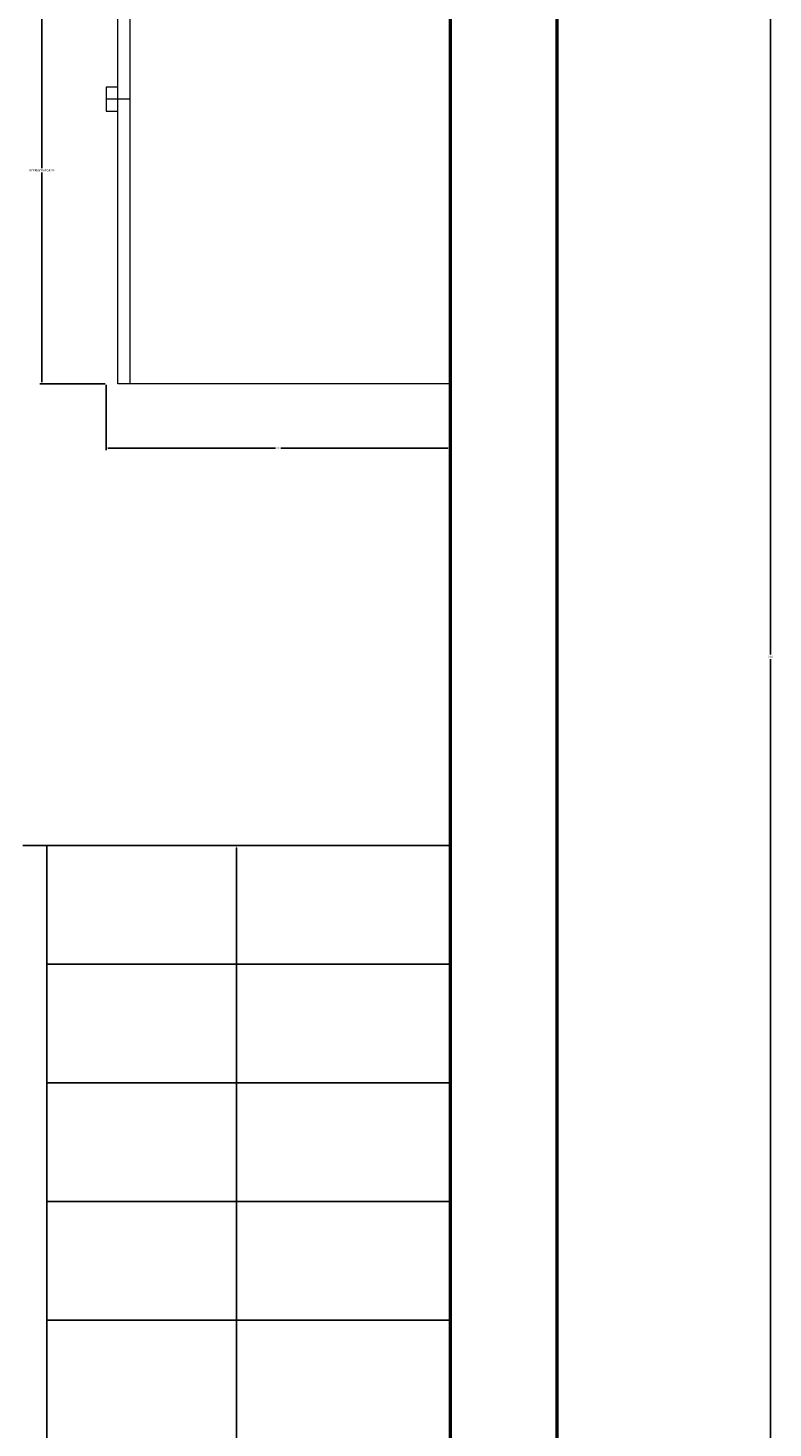
# Model space of a CAD drawing. Units: inches. Extents: x 2621 to 2849, y 2066 to 2463.
# Tile 12 of 28: x 2786 to 2849, y 2199 to 2317. Entities that reach past the tile are written whole.
import ezdxf

# ---------------------------------------------------------------- set-up
doc = ezdxf.new("R2010")
doc.units = ezdxf.units.IN
for name, color, linetype, lineweight in [('A-ANNO-DIMS', 2, 'Continuous', 18), ('A-EQPM', 8, 'Continuous', 18), ('A-FLOR-STRS', 7, 'Continuous', 25), ('A-WALL', 7, 'Continuous', 50)]:
    doc.layers.add(name, color=color, linetype=linetype, lineweight=lineweight)
doc.styles.get("Standard").update_dxf_attribs({"font": 'arial.ttf'})
doc.dimstyles.get("Standard").update_dxf_attribs({"dimtxt": 0.18, "dimasz": 0.18, "dimexe": 0.18, "dimexo": 0.0625, "dimgap": 0.09, "dimtad": 0, "dimtih": 1, "dimtoh": 1, "dimdec": 4, "dimzin": 0, "dimdsep": 46, "dimtxsty": 'Standard', "dimcen": 0.09, "dimadec": 0, "dimazin": 0, "dimtfac": 1, "dimtdec": 4, "dimtofl": 0, "dimtmove": 0, "dimatfit": 3, "dimfxl": 1, "dimtolj": 1, "dimtzin": 0, "dimarcsym": 0})

# ---------------------------------------------------------------- blocks, each defined once
blk = doc.blocks.new('Refrigerator-2 door - 36 in top')
for p, q in [((0, -26.999999), (36, -26.999999)), ((12, -26.999999), (12, -28.999999)), ((11, -27.999999), (11, -28.999999)), ((13, -28.999999), (13, -27.999999)), ((11, -28.999999), (13, -28.999999))]:
    blk.add_line(p, q)
blk.add_lwpolyline([(0, -27.999999), (0, 0), (36, 0), (36, -27.999999)], close=True)
blk = doc.blocks.new('*D17')
at = {"layer": 'A-ANNO-DIMS', "color": 0, "lineweight": -2, "transparency": 16777216}
for p, q in [((2792.81, 2323.37), (2787.29, 2323.37)), ((2787.47, 2323.19), (2787.47, 2305.56)), ((2787.47, 2287.55), (2787.47, 2305.19)), ((2792.81, 2287.37), (2787.29, 2287.37))]:
    blk.add_line(p, q, dxfattribs=at)
at = {"layer": 'A-ANNO-DIMS', "color": 0, "transparency": 16777216}
for points in [[(2787.44, 2323.19), (2787.5, 2323.19), (2787.47, 2323.37)], [(2787.44, 2287.55), (2787.5, 2287.55), (2787.47, 2287.37)]]:
    blk.add_solid(points, dxfattribs=at)
at = {"layer": 'Defpoints', "color": 0, "transparency": 16777216}
for p in [(2792.87, 2323.37), (2787.47, 2287.37), (2792.87, 2287.37)]:
    blk.add_point(p, dxfattribs=at)
at = {"layer": 'A-ANNO-DIMS', "color": 0, "transparency": 16777216, "insert": (2787.47, 2305.37), "char_height": 0.18, "attachment_point": 5}
blk.add_mtext('\\A1;REFRIGERATOR 36', dxfattribs=at)
blk = doc.blocks.new('*D18')
at = {"layer": 'A-ANNO-DIMS', "color": 0, "lineweight": -2, "transparency": 16777216}
for p, q in [((2792.87, 2287.31), (2792.87, 2281.79)), ((2821.87, 2287.31), (2821.87, 2281.79)), ((2793.05, 2281.97), (2807.15, 2281.97)), ((2821.69, 2281.97), (2807.59, 2281.97))]:
    blk.add_line(p, q, dxfattribs=at)
at = {"layer": 'A-ANNO-DIMS', "color": 0, "transparency": 16777216}
for points in [[(2793.05, 2282), (2793.05, 2281.94), (2792.87, 2281.97)], [(2821.69, 2282), (2821.69, 2281.94), (2821.87, 2281.97)]]:
    blk.add_solid(points, dxfattribs=at)
at = {"layer": 'Defpoints', "color": 0, "transparency": 16777216}
for p in [(2792.87, 2287.37), (2821.87, 2287.37), (2821.87, 2281.97)]:
    blk.add_point(p, dxfattribs=at)
at = {"layer": 'A-ANNO-DIMS', "color": 0, "transparency": 16777216, "insert": (2807.37, 2281.97), "char_height": 0.18, "attachment_point": 5}
blk.add_mtext('\\A1;29', dxfattribs=at)
blk = doc.blocks.new('*D36')
at = {"layer": 'A-ANNO-DIMS', "color": 0, "lineweight": -2, "transparency": 16777216}
for p, q in [((2830.93, 2444.37), (2849.05, 2444.37)), ((2848.87, 2444.19), (2848.87, 2264.56)), ((2848.87, 2084.55), (2848.87, 2264.19)), ((2830.93, 2084.37), (2849.05, 2084.37))]:
    blk.add_line(p, q, dxfattribs=at)
at = {"layer": 'A-ANNO-DIMS', "color": 0, "transparency": 16777216}
for points in [[(2848.84, 2444.19), (2848.9, 2444.19), (2848.87, 2444.37)], [(2848.84, 2084.55), (2848.9, 2084.55), (2848.87, 2084.37)]]:
    blk.add_solid(points, dxfattribs=at)
at = {"layer": 'Defpoints', "color": 0, "transparency": 16777216}
for p in [(2830.87, 2444.37), (2848.87, 2444.37), (2830.87, 2084.37)]:
    blk.add_point(p, dxfattribs=at)
at = {"layer": 'A-ANNO-DIMS', "color": 0, "transparency": 16777216, "insert": (2848.87, 2264.37), "char_height": 0.18, "attachment_point": 5}
blk.add_mtext('\\A1;360', dxfattribs=at)
blk = doc.blocks.new('*D58')
at = {"layer": 'A-ANNO-DIMS', "color": 0, "lineweight": -2, "transparency": 16777216}
for p, q in [((2821.81, 2248.46), (2803.69, 2248.46)), ((2803.87, 2248.28), (2803.87, 2193.64)), ((2803.87, 2138.64), (2803.87, 2193.28)), ((2821.81, 2138.46), (2803.69, 2138.46))]:
    blk.add_line(p, q, dxfattribs=at)
at = {"layer": 'A-ANNO-DIMS', "color": 0, "transparency": 16777216}
for points in [[(2803.84, 2248.28), (2803.9, 2248.28), (2803.87, 2248.46)], [(2803.84, 2138.64), (2803.9, 2138.64), (2803.87, 2138.46)]]:
    blk.add_solid(points, dxfattribs=at)
at = {"layer": 'Defpoints', "color": 0, "transparency": 16777216}
for p in [(2803.87, 2248.46), (2821.87, 2248.46), (2821.87, 2138.46)]:
    blk.add_point(p, dxfattribs=at)
at = {"layer": 'A-ANNO-DIMS', "color": 0, "transparency": 16777216, "insert": (2803.87, 2193.46), "char_height": 0.18, "attachment_point": 5}
blk.add_mtext('\\A1;110', dxfattribs=at)

msp = doc.modelspace()

# ---------------------------------------------------------------- linework, layer by layer
at = {"layer": 'A-FLOR-STRS'}
for p, q in [((2821.8701, 2248.4598), (2785.8701, 2248.4598)), ((2787.8701, 2248.4598), (2787.8701, 2158.4598)), ((2821.8701, 2238.4598), (2787.8701, 2238.4598)), ((2821.8701, 2228.4598), (2787.8701, 2228.4598)), ((2821.8701, 2218.4598), (2787.8701, 2218.4598)), ((2821.8701, 2208.4598), (2787.8701, 2208.4598))]:
    msp.add_line(p, q, dxfattribs=at)
at = {"layer": 'A-WALL'}
msp.add_line((2821.8701, 2371.3746), (2821.8701, 2093.3746), dxfattribs=at)
msp.add_lwpolyline([(2761.8701, 2084.3746), (2638.8701, 2084.3746), (2638.8701, 2444.3746), (2830.8701, 2444.3746), (2830.8701, 2084.3746), (2797.8701, 2084.3746)], dxfattribs=at)

# ---------------------------------------------------------------- block references
at = {"layer": 'A-EQPM', "rotation": 270}
msp.add_blockref('Refrigerator-2 door - 36 in top', (2821.8701, 2323.3746), dxfattribs=at)

# ---------------------------------------------------------------- dimensions: what is measured, and where the dimension line sits
at = {"layer": 'A-ANNO-DIMS'}
for base, p1, p2, picture, middle in [((2848.8736, 2444.3746), (2830.8701, 2084.3746), (2830.8701, 2444.3746), '*D36', (2848.8736, 2264.3746)), ((2803.8666, 2248.4598), (2821.8701, 2138.4598), (2821.8701, 2248.4598), '*D58', (2803.8666, 2193.4598))]:
    dim = msp.add_linear_dim(base=base, p1=p1, p2=p2, angle=90, dimstyle='Standard', override={"dimdec": 0, "dimlfac": 1, "dimrnd": 0, "dimzin": 0, "dimdsep": 46, "dimlunit": 2}, dxfattribs=at)
    dim.commit()
    dim.dimension.update_dxf_attribs({"geometry": picture, "text_midpoint": middle})
dim = msp.add_linear_dim(base=(2787.4701, 2287.3746), p1=(2792.8701, 2323.3746), p2=(2792.8701, 2287.3746), angle=270, text='REFRIGERATOR <>', dimstyle='Standard', override={"dimdec": 0, "dimlfac": 1, "dimrnd": 0, "dimzin": 0, "dimdsep": 46, "dimlunit": 2}, dxfattribs=at)
dim.commit()
dim.dimension.update_dxf_attribs({"geometry": '*D17', "text_midpoint": (2787.4701, 2305.3746)})
dim = msp.add_linear_dim(base=(2821.8701, 2281.9746), p1=(2792.8701, 2287.3746), p2=(2821.8701, 2287.3746), dimstyle='Standard', override={"dimdec": 0, "dimlfac": 1, "dimrnd": 0, "dimzin": 0, "dimdsep": 46, "dimlunit": 2}, dxfattribs=at)
dim.commit()
dim.dimension.update_dxf_attribs({"geometry": '*D18', "text_midpoint": (2807.3701, 2281.9746)})

doc.saveas('drawing.dxf')
